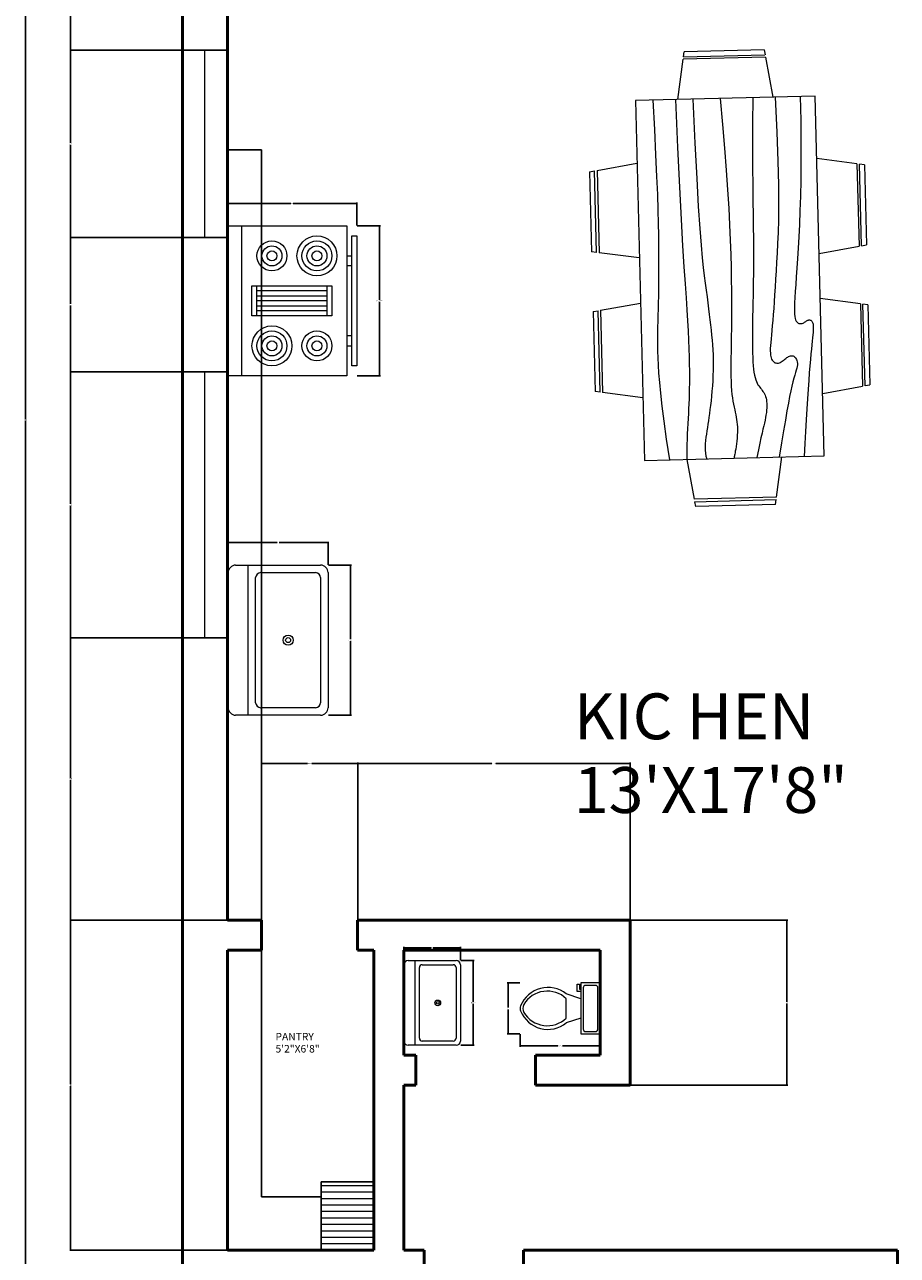
# Model space of a CAD drawing. Units: inches. Extents: x 2208 to 4689, y 1219 to 3512.
# Tile 2 of 5: x 2208 to 2382, y 1383 to 1629. Entities that reach past the tile are written whole.
import ezdxf

# ---------------------------------------------------------------- set-up
doc = ezdxf.new("R2010")
doc.units = ezdxf.units.IN
for name, color, linetype, lineweight in [('A-ANNO-DIMS', 2, 'Continuous', 18), ('A-AREA-IDEN', 7, 'Continuous', 18), ('A-EQPM', 8, 'Continuous', 20), ('A-FLOR-CASE', 9, 'Continuous', 25), ('A-FLOR-FIXT', 9, 'Continuous', 20), ('A-FLOR-PATT', 8, 'Continuous', 13), ('A-FURN', 8, 'Continuous', 18), ('A-GLAZ', 4, 'Continuous', 18), ('A-WALL', 7, 'Continuous', 50)]:
    doc.layers.add(name, color=color, linetype=linetype, lineweight=lineweight)
doc.styles.get("Standard").update_dxf_attribs({"font": 'arial.ttf'})
doc.dimstyles.get("Standard").update_dxf_attribs({"dimtxt": 0.18, "dimasz": 0.18, "dimexe": 0.18, "dimexo": 0.0625, "dimgap": 0.09, "dimtad": 0, "dimtih": 1, "dimtoh": 1, "dimdec": 4, "dimzin": 0, "dimdsep": 46, "dimtxsty": 'Standard', "dimcen": 0.09, "dimadec": 0, "dimazin": 0, "dimtfac": 1, "dimtdec": 4, "dimtofl": 0, "dimtmove": 0, "dimatfit": 3, "dimfxl": 1, "dimtolj": 1, "dimtzin": 0, "dimarcsym": 0})

# ---------------------------------------------------------------- blocks, each defined once
blk = doc.blocks.new('Sink-single - 30 in top')
blk.add_line((-15, -3.999996), (15, -3.999996))
for points in [[(-13.5, 0), (13.5, 0)], [(-15, -18.499996), (-15, -1.5)], [(15, -1.5), (15, -18.499996)], [(-13.5, -17.499996), (-13.5, -6.499996)], [(-12.5, -5.499996), (12.5, -5.499996)], [(13.5, -6.499996), (13.5, -17.499996)], [(12.5, -18.499996), (-12.5, -18.499996)], [(13.5, -19.999996), (-13.5, -19.999996)]]:
    blk.add_lwpolyline(points)
for radius in [1, 0.5]:
    blk.add_circle((0, -11.999996), radius)
for centre, radius, start, end in [((-13.5, -1.5), 1.5, 90, 180), ((13.5, -1.5), 1.5, 0, 90), ((-12.5, -6.499996), 1, 90, 180), ((12.5, -6.499996), 1, 0, 90), ((-13.5, -18.499996), 1.5, 180, 270), ((-12.5, -17.499996), 1, 180, 270), ((12.5, -17.499996), 1, 270, 0), ((13.5, -18.499996), 1.5, 270, 0)]:
    blk.add_arc(centre, radius, start, end)
blk = doc.blocks.new('Range-Oven - 30 in top')
for p, q in [((0, -3), (30, -3)), ((12, -6), (18, -6)), ((13, -20), (13, -6)), ((14, -6), (14, -20)), ((15, -20), (15, -6)), ((16, -6), (16, -20)), ((17, -20), (17, -6)), ((18, -20), (12, -20)), ((6, -24), (6, -25)), ((8, -25), (8, -24)), ((22, -25), (22, -24)), ((24, -24), (24, -25))]:
    blk.add_line(p, q)
for points in [[(0, -24), (0, 0), (30, 0), (30, -24)], [(12, -21), (12, -5), (18, -5), (18, -21)], [(2, -26), (2, -25), (28, -25), (28, -26)]]:
    blk.add_lwpolyline(points, close=True)
for centre, radius in [((6, -9), 4), ((6, -9), 3), ((6, -9), 2), ((24, -9), 3), ((24, -9), 2), ((6, -9), 1), ((24, -9), 1), ((24, -18), 4), ((6, -18), 3), ((6, -18), 2), ((6, -18), 1), ((24, -18), 3), ((24, -18), 2), ((24, -18), 1)]:
    blk.add_circle(centre, radius)
blk = doc.blocks.new('Toilet - top')
for p, q in [((9.5, -6), (9.5, -2)), ((-10, -8.5), (-8, -8.5)), ((-10, -9.5), (-10, -8.5)), ((-7, -9.5), (-10, -9.5)), ((-8, -8.5), (-8, -8)), ((-7, -8), (-7, -9.5)), ((-4, -8), (-6, -14)), ((4, -8), (6, -14)), ((4, -14), (-4, -14))]:
    blk.add_line(p, q)
blk.add_lwpolyline([(10.5, -8), (10.5, 0), (-10.5, 0), (-10.5, -8)], close=True)
for points in [[(-9.5, -2), (-9.5, -6)], [(8.5, -1), (-8.5, -1)], [(-8.5, -7), (8.5, -7)]]:
    blk.add_lwpolyline(points)
for centre, radius, start, end in [((-8.62, -1.88), 0.884, 81.8699, 188.1301), ((8.62, -1.88), 0.884, 351.8699, 98.1301), ((-8.62, -6.12), 0.884, 171.8699, 278.1301), ((8.62, -6.12), 0.884, 261.8699, 8.1301), ((3.52, -21.58), 12.17, 141.4691, 247.9714), ((4.2, -21.82), 11.33, 136.3677, 238.9468), ((-3.52, -21.58), 12.17, 292.0284, 38.5307), ((-4.2, -21.82), 11.33, 301.053, 43.6321), ((0, -27.88), 4, 245.7318, 294.2682), ((0, -29), 4, 254.8605, 285.1395)]:
    blk.add_arc(centre, radius, start, end)
blk = doc.blocks.new('Dining Set - 36 x 72 in.')
for p, q in [((-22, 27.5), (-22.1562, 26.50042)), ((-22, 27.5), (-6, 27.5)), ((-5.8437, 26.49966), (-6, 27.5)), ((6, 27.5), (5.8438, 26.50042)), ((6, 27.5), (22, 27.5)), ((22.1563, 26.49966), (22, 27.5)), ((-22.2343, 26.00059), (-23.4847, 17.99762)), ((-22.2304, 26), (-5.7608, 26)), ((-5.8416, 26.5), (-22.1534, 26.5)), ((-4.5152, 17.99762), (-5.7655, 25.99926)), ((5.7657, 26.00059), (4.5153, 17.99762)), ((5.7696, 26), (22.2392, 26)), ((22.1584, 26.5), (5.8466, 26.5)), ((23.4848, 17.99762), (22.2345, 25.99926)), ((36, 18), (-36, 18)), ((-36, 18), (-36, -18)), ((36, -18), (36, 18)), ((-45.5, 8), (-44.5004, 8.15617)), ((-45.5, 8), (-45.5, -8)), ((-44.5, -8.15843), (-44.5, 8.15338)), ((-44.0006, 8.23428), (-35.9976, 9.48474)), ((-44, 8.23041), (-44, -8.23915)), ((44.0006, 8.23428), (35.9976, 9.48474)), ((44, 8.23041), (44, -8.23915)), ((44.5, -8.15843), (44.5, 8.15338)), ((45.5, 8), (44.5005, 8.15617)), ((45.5, 8), (45.5, -8)), ((-44.4997, -8.15631), (-45.5, -8)), ((-35.9976, -9.48476), (-43.9993, -8.2345)), ((35.9976, -9.48476), (43.9993, -8.2345)), ((44.4997, -8.15631), (45.5, -8)), ((-36, -18), (36, -18)), ((-22.2343, -26.0006), (-23.4847, -17.99762)), ((-4.5152, -17.99762), (-5.7655, -25.99928)), ((5.7657, -26.0006), (4.5153, -17.99762)), ((23.4848, -17.99762), (22.2345, -25.99928)), ((-22.2304, -26), (-5.7608, -26)), ((-22, -27.5), (-22.1562, -26.50044)), ((-5.8416, -26.5), (-22.1534, -26.5)), ((-5.8437, -26.49967), (-6, -27.5)), ((5.7696, -26), (22.2392, -26)), ((6, -27.5), (5.8438, -26.50044)), ((22.1584, -26.5), (5.8466, -26.5)), ((22.1563, -26.49967), (22, -27.5)), ((-22, -27.5), (-6, -27.5)), ((6, -27.5), (22, -27.5))]:
    blk.add_line(p, q)
for points in [[(-36, 15), (-31.1772, 14.97754), (-26.8079, 14.91406), (-22.8538, 14.81543), (-19.276, 14.6875), (-16.0362, 14.53613), (-13.0957, 14.36718), (-10.4159, 14.18652), (-7.9583, 14), (-5.6904, 13.81315), (-3.6035, 13.63021), (-1.6954, 13.45508), (0.0365, 13.29166), (1.5945, 13.14388), (2.9811, 13.01562), (4.1988, 12.9108), (5.25, 12.83333), (6.1393, 12.78613), (6.8802, 12.76823), (7.4883, 12.77767), (7.9792, 12.8125), (8.3685, 12.87077), (8.6719, 12.95052), (8.9049, 13.0498), (9.0833, 13.16666), (9.2205, 13.29899), (9.3216, 13.44401), (9.3895, 13.59879), (9.4271, 13.76041), (9.4373, 13.92594), (9.4232, 14.09245), (9.3875, 14.257), (9.3333, 14.41666), (9.2638, 14.56917), (9.1836, 14.71484), (9.0975, 14.85465), (9.0104, 14.98958), (8.9272, 15.1206), (8.8529, 15.2487), (8.7922, 15.37483), (8.75, 15.5), (8.7305, 15.62467), (8.7344, 15.74739), (8.7617, 15.86621), (8.8125, 15.97916), (8.8867, 16.08431), (8.9844, 16.17968), (9.1055, 16.26334), (9.25, 16.33333), (9.4189, 16.38802), (9.6172, 16.42708), (9.8506, 16.45052), (10.125, 16.45833), (10.4463, 16.45052), (10.8203, 16.42708), (11.2529, 16.38802), (11.75, 16.33333), (12.3184, 16.26318), (12.9694, 16.17838), (13.7151, 16.07991), (14.5677, 15.96875), (15.5395, 15.84586), (16.6426, 15.71224), (17.8893, 15.56884), (19.2917, 15.41666), (20.859, 15.25667), (22.5879, 15.08984), (24.4721, 14.91715), (26.5052, 14.73958), (28.6809, 14.5581), (30.9929, 14.3737), (33.4347, 14.18733), (36, 14)], [(-36, 10), (-28.9766, 10.14274), (-23.1725, 10.20442), (-18.4241, 10.19775), (-14.5677, 10.13541), (-11.4399, 10.03011), (-8.877, 9.89453), (-6.7154, 9.74137), (-4.7917, 9.58333), (-2.9698, 9.43082), (-1.2246, 9.28515), (0.4415, 9.14534), (2.026, 9.01041), (3.5266, 8.87939), (4.9408, 8.7513), (6.266, 8.62516), (7.5, 8.5), (8.6411, 8.37549), (9.6914, 8.2539), (10.6538, 8.13818), (11.5312, 8.03125), (12.3267, 7.93603), (13.043, 7.85547), (13.6831, 7.79248), (14.25, 7.75), (14.7471, 7.7303), (15.1797, 7.73307), (15.5537, 7.75732), (15.875, 7.80208), (16.1494, 7.86637), (16.3828, 7.94922), (16.5811, 8.04964), (16.75, 8.16666), (16.8944, 8.29915), (17.0143, 8.44531), (17.1089, 8.60319), (17.1771, 8.77083), (17.218, 8.94629), (17.2305, 9.1276), (17.2137, 9.31282), (17.1667, 9.5), (17.0895, 9.6875), (16.987, 9.875), (16.8649, 10.0625), (16.7292, 10.25), (16.5856, 10.4375), (16.4401, 10.625), (16.2985, 10.8125), (16.1667, 11), (16.05, 11.18733), (15.9518, 11.3737), (15.8752, 11.5581), (15.8229, 11.73958), (15.798, 11.91715), (15.8034, 12.08984), (15.842, 12.25667), (15.9167, 12.41666), (16.0295, 12.56836), (16.1784, 12.70833), (16.3605, 12.83268), (16.5729, 12.9375), (16.8127, 13.01888), (17.0768, 13.07291), (17.3625, 13.0957), (17.6667, 13.08333), (17.9894, 13.03312), (18.3418, 12.94726), (18.7382, 12.82918), (19.1927, 12.68229), (19.7195, 12.51001), (20.3327, 12.31575), (21.0465, 12.10294), (21.875, 11.875), (22.8357, 11.63354), (23.959, 11.37304), (25.2786, 11.08618), (26.8282, 10.76562), (28.6414, 10.40405), (30.752, 9.99414), (33.1936, 9.52856), (36, 9)], [(-36, 5.5), (-30.7157, 5.3348), (-26.069, 5.20963), (-21.9946, 5.11767), (-18.4271, 5.05208), (-15.3009, 5.00602), (-12.5508, 4.97265), (-10.1112, 4.94515), (-7.9167, 4.91666), (-5.909, 4.88167), (-4.0586, 4.83984), (-2.3429, 4.79215), (-0.7396, 4.73958), (0.7739, 4.6831), (2.22, 4.6237), (3.6213, 4.56233), (5, 4.5), (6.373, 4.43782), (7.7344, 4.3776), (9.0723, 4.32129), (10.375, 4.27083), (11.6309, 4.22819), (12.8281, 4.19531), (13.9551, 4.17415), (15, 4.16666), (15.954, 4.17448), (16.819, 4.19791), (17.6001, 4.23698), (18.3021, 4.29166), (18.9299, 4.36198), (19.4883, 4.44791), (19.9823, 4.54948), (20.4167, 4.66666), (20.7969, 4.79899), (21.1302, 4.94401), (21.4245, 5.09879), (21.6875, 5.26041), (21.9271, 5.42594), (22.1511, 5.59245), (22.3672, 5.757), (22.5834, 5.91666), (22.8065, 6.06868), (23.0404, 6.21093), (23.2879, 6.34147), (23.5521, 6.45833), (23.8358, 6.55957), (24.142, 6.64323), (24.4735, 6.70735), (24.8334, 6.75), (25.2235, 6.76969), (25.642, 6.76692), (26.0858, 6.74267), (26.5521, 6.69791), (27.0379, 6.63362), (27.5404, 6.55078), (28.0565, 6.45036), (28.5834, 6.33333), (29.1242, 6.19987), (29.7071, 6.04687), (30.3661, 5.87044), (31.1354, 5.66666), (32.0493, 5.43164), (33.142, 5.16146), (34.4475, 4.85221), (36, 4.5)], [(-36, -1), (-30.7915, -0.6591), (-26.0195, -0.38216), (-21.6519, -0.16284), (-17.6563, 0.00521), (-14.0005, 0.12833), (-10.6523, 0.21289), (-7.5796, 0.26522), (-4.75, 0.29166), (-2.134, 0.29793), (0.2878, 0.28711), (2.5317, 0.26163), (4.6146, 0.22396), (6.5529, 0.17651), (8.3633, 0.12174), (10.0623, 0.06209), (11.6667, 0), (13.1899, -0.06201), (14.6341, -0.1211), (15.9982, -0.17432), (17.2813, -0.21875), (18.4823, -0.25147), (19.6003, -0.26953), (20.6343, -0.27002), (21.5834, -0.25), (22.4481, -0.20768), (23.2357, -0.14584), (23.9549, -0.06836), (24.6146, 0.02083), (25.2235, 0.11784), (25.7904, 0.21875), (26.3241, 0.31966), (26.8334, 0.41666), (27.3265, 0.50618), (27.8099, 0.58593), (28.2894, 0.65397), (28.7709, 0.70833), (29.2601, 0.74707), (29.763, 0.76823), (30.2855, 0.76985), (30.8334, 0.75), (31.4088, 0.70784), (31.9994, 0.64713), (32.589, 0.57275), (33.1615, 0.48958), (33.7008, 0.4025), (34.1908, 0.3164), (34.6153, 0.23616), (34.9584, 0.16666), (35.2099, 0.11165), (35.3848, 0.07031), (35.504, 0.04069), (35.5886, 0.02083), (35.6594, 0.00879), (35.7377, 0.0026), (35.8442, 0.00032), (36, 0)], [(-36, -6.5), (-27.1843, -6.31267), (-20.084, -6.1263), (-14.469, -5.9419), (-10.1094, -5.76042), (-6.7752, -5.58285), (-4.2363, -5.41016), (-2.2629, -5.24333), (-0.625, -5.08334), (0.8708, -4.93099), (2.2715, -4.78646), (3.5872, -4.64974), (4.8281, -4.52084), (6.0046, -4.39974), (7.127, -4.28646), (8.2053, -4.18099), (9.25, -4.08334), (10.2705, -3.99382), (11.2734, -3.91407), (12.2647, -3.84603), (13.25, -3.79167), (14.2354, -3.75293), (15.2266, -3.73177), (16.2295, -3.73015), (17.25, -3.75), (18.2912, -3.79248), (19.3451, -3.85547), (20.4009, -3.93604), (21.4479, -4.03125), (22.4754, -4.13819), (23.4727, -4.25391), (24.4289, -4.37549), (25.3334, -4.5), (26.1785, -4.62492), (26.9694, -4.74935), (27.7145, -4.87281), (28.4219, -4.99479), (29.1, -5.11483), (29.7572, -5.23242), (30.4016, -5.34709), (31.0417, -5.45834), (31.6837, -5.56437), (32.3262, -5.65821), (32.9658, -5.73153), (33.599, -5.77604), (34.2224, -5.78345), (34.8327, -5.74545), (35.4264, -5.65373), (36, -5.5)], [(-36, -10), (-26.4022, -9.81299), (-18.4675, -9.62891), (-11.9839, -9.45069), (-6.7396, -9.28125), (-2.5226, -9.12354), (0.8789, -8.98047), (3.6769, -8.85498), (6.0833, -8.75), (8.2767, -8.66765), (10.3021, -8.60677), (12.1712, -8.56543), (13.8958, -8.54167), (15.4876, -8.53353), (16.9583, -8.53907), (18.3197, -8.55632), (19.5834, -8.58334), (20.7616, -8.61841), (21.8685, -8.66081), (22.9188, -8.71004), (23.9271, -8.76563), (24.9081, -8.82707), (25.8763, -8.89388), (26.8465, -8.96558), (27.8334, -9.04167), (28.8474, -9.12118), (29.8828, -9.20117), (30.93, -9.27824), (31.9792, -9.34896), (33.0205, -9.40991), (34.0443, -9.45768), (35.0407, -9.48885), (36, -9.5)], [(-36, -14.5), (-30.0881, -14.33513), (-25.0332, -14.21224), (-20.7312, -14.12647), (-17.0781, -14.07292), (-13.97, -14.04671), (-11.3027, -14.04297), (-8.9724, -14.05681), (-6.875, -14.08334), (-4.9224, -14.11833), (-3.0905, -14.16016), (-1.3709, -14.20785), (0.2448, -14.26042), (1.7647, -14.3169), (3.1973, -14.3763), (4.5507, -14.43767), (5.8333, -14.5), (7.0554, -14.5621), (8.235, -14.62175), (9.3922, -14.67652), (10.5469, -14.72396), (11.7192, -14.76164), (12.929, -14.78711), (14.1965, -14.79794), (15.5417, -14.79167), (16.9933, -14.76424), (18.6152, -14.70508), (20.4804, -14.60197), (22.6615, -14.44271), (25.2312, -14.21509), (28.2624, -13.9069), (31.8277, -13.50594), (36, -13)]]:
    blk.add_lwpolyline(points)
blk = doc.blocks.new('*D22')
at = {"layer": 'A-ANNO-DIMS', "color": 0, "lineweight": -2, "transparency": 16777216}
for p, q in [((2268.33, 1521.37), (2272.94, 1521.37)), ((2272.76, 1521.19), (2272.76, 1506.55)), ((2272.76, 1491.55), (2272.76, 1506.18)), ((2268.33, 1491.37), (2272.94, 1491.37))]:
    blk.add_line(p, q, dxfattribs=at)
at = {"layer": 'A-ANNO-DIMS', "color": 0, "transparency": 16777216}
for points in [[(2272.73, 1521.19), (2272.79, 1521.19), (2272.76, 1521.37)], [(2272.73, 1491.55), (2272.79, 1491.55), (2272.76, 1491.37)]]:
    blk.add_solid(points, dxfattribs=at)
at = {"layer": 'Defpoints', "color": 0, "transparency": 16777216}
for p in [(2268.26, 1521.37), (2272.76, 1521.37), (2268.26, 1491.37)]:
    blk.add_point(p, dxfattribs=at)
at = {"layer": 'A-ANNO-DIMS', "color": 0, "transparency": 16777216, "insert": (2272.76, 1506.37), "char_height": 0.18, "attachment_point": 5}
blk.add_mtext('\\A1;SINK 30', dxfattribs=at)
blk = doc.blocks.new('*D23')
at = {"layer": 'A-ANNO-DIMS', "color": 0, "lineweight": -2, "transparency": 16777216}
for p, q in [((2248.26, 1521.43), (2248.26, 1526.05)), ((2248.44, 1525.87), (2258.04, 1525.87)), ((2268.08, 1525.87), (2258.48, 1525.87)), ((2268.26, 1521.43), (2268.26, 1526.05))]:
    blk.add_line(p, q, dxfattribs=at)
at = {"layer": 'A-ANNO-DIMS', "color": 0, "transparency": 16777216}
for points in [[(2248.44, 1525.9), (2248.44, 1525.84), (2248.26, 1525.87)], [(2268.08, 1525.9), (2268.08, 1525.84), (2268.26, 1525.87)]]:
    blk.add_solid(points, dxfattribs=at)
at = {"layer": 'Defpoints', "color": 0, "transparency": 16777216}
for p in [(2248.26, 1525.87), (2248.26, 1521.37), (2268.26, 1521.37)]:
    blk.add_point(p, dxfattribs=at)
at = {"layer": 'A-ANNO-DIMS', "color": 0, "transparency": 16777216, "insert": (2258.26, 1525.87), "char_height": 0.18, "attachment_point": 5}
blk.add_mtext('\\A1;20', dxfattribs=at)
blk = doc.blocks.new('*D24')
at = {"layer": 'A-ANNO-DIMS', "color": 0, "lineweight": -2, "transparency": 16777216}
for p, q in [((2294.78, 1442.31), (2297.44, 1442.31)), ((2297.26, 1442.13), (2297.26, 1434.01)), ((2297.26, 1425.53), (2297.26, 1433.65)), ((2294.78, 1425.35), (2297.44, 1425.35))]:
    blk.add_line(p, q, dxfattribs=at)
at = {"layer": 'A-ANNO-DIMS', "color": 0, "transparency": 16777216}
for points in [[(2297.23, 1442.13), (2297.29, 1442.13), (2297.26, 1442.31)], [(2297.23, 1425.53), (2297.29, 1425.53), (2297.26, 1425.35)]]:
    blk.add_solid(points, dxfattribs=at)
at = {"layer": 'Defpoints', "color": 0, "transparency": 16777216}
for p in [(2294.71, 1442.31), (2297.26, 1442.31), (2294.71, 1425.35)]:
    blk.add_point(p, dxfattribs=at)
at = {"layer": 'A-ANNO-DIMS', "color": 0, "transparency": 16777216, "insert": (2297.26, 1433.83), "char_height": 0.18, "attachment_point": 5}
blk.add_mtext('\\A1;SINK 17', dxfattribs=at)
blk = doc.blocks.new('*D25')
at = {"layer": 'A-ANNO-DIMS', "color": 0, "lineweight": -2, "transparency": 16777216}
for p, q in [((2283.4, 1442.38), (2283.4, 1445.04)), ((2294.71, 1442.38), (2294.71, 1445.04)), ((2283.58, 1444.86), (2288.87, 1444.86)), ((2294.53, 1444.86), (2289.25, 1444.86))]:
    blk.add_line(p, q, dxfattribs=at)
at = {"layer": 'A-ANNO-DIMS', "color": 0, "transparency": 16777216}
for points in [[(2283.58, 1444.89), (2283.58, 1444.83), (2283.4, 1444.86)], [(2294.53, 1444.89), (2294.53, 1444.83), (2294.71, 1444.86)]]:
    blk.add_solid(points, dxfattribs=at)
at = {"layer": 'Defpoints', "color": 0, "transparency": 16777216}
for p in [(2283.4, 1444.86), (2283.4, 1442.31), (2294.71, 1442.31)]:
    blk.add_point(p, dxfattribs=at)
at = {"layer": 'A-ANNO-DIMS', "color": 0, "transparency": 16777216, "insert": (2289.06, 1444.86), "char_height": 0.18, "attachment_point": 5}
blk.add_mtext('\\A1;11', dxfattribs=at)
blk = doc.blocks.new('*D28')
at = {"layer": 'A-ANNO-DIMS', "color": 0, "lineweight": -2, "transparency": 16777216}
for p, q in [((2274.09, 1589.22), (2278.71, 1589.22)), ((2278.53, 1589.04), (2278.53, 1574.41)), ((2278.53, 1559.4), (2278.53, 1574.04)), ((2274.09, 1559.22), (2278.71, 1559.22))]:
    blk.add_line(p, q, dxfattribs=at)
at = {"layer": 'A-ANNO-DIMS', "color": 0, "transparency": 16777216}
for points in [[(2278.5, 1589.04), (2278.56, 1589.04), (2278.53, 1589.22)], [(2278.5, 1559.4), (2278.56, 1559.4), (2278.53, 1559.22)]]:
    blk.add_solid(points, dxfattribs=at)
at = {"layer": 'Defpoints', "color": 0, "transparency": 16777216}
for p in [(2274.03, 1589.22), (2278.53, 1589.22), (2274.03, 1559.22)]:
    blk.add_point(p, dxfattribs=at)
at = {"layer": 'A-ANNO-DIMS', "color": 0, "transparency": 16777216, "insert": (2278.53, 1574.22), "char_height": 0.18, "attachment_point": 5}
blk.add_mtext('\\A1;RANGE 30', dxfattribs=at)
blk = doc.blocks.new('*D29')
at = {"layer": 'A-ANNO-DIMS', "color": 0, "lineweight": -2, "transparency": 16777216}
for p, q in [((2248.03, 1589.29), (2248.03, 1593.9)), ((2248.21, 1593.72), (2260.81, 1593.72)), ((2273.85, 1593.72), (2261.25, 1593.72)), ((2274.03, 1589.29), (2274.03, 1593.9))]:
    blk.add_line(p, q, dxfattribs=at)
at = {"layer": 'A-ANNO-DIMS', "color": 0, "transparency": 16777216}
for points in [[(2248.21, 1593.75), (2248.21, 1593.69), (2248.03, 1593.72)], [(2273.85, 1593.75), (2273.85, 1593.69), (2274.03, 1593.72)]]:
    blk.add_solid(points, dxfattribs=at)
at = {"layer": 'Defpoints', "color": 0, "transparency": 16777216}
for p in [(2248.03, 1593.72), (2248.03, 1589.22), (2274.03, 1589.22)]:
    blk.add_point(p, dxfattribs=at)
at = {"layer": 'A-ANNO-DIMS', "color": 0, "transparency": 16777216, "insert": (2261.03, 1593.72), "char_height": 0.18, "attachment_point": 5}
blk.add_mtext('\\A1;26', dxfattribs=at)
blk = doc.blocks.new('*D30')
at = {"layer": 'A-ANNO-DIMS', "color": 0, "lineweight": -2, "transparency": 16777216}
for p, q in [((2306.67, 1427.56), (2306.67, 1425.04)), ((2306.85, 1425.22), (2314.21, 1425.22)), ((2322.51, 1425.22), (2315.15, 1425.22)), ((2322.69, 1427.56), (2322.69, 1425.04))]:
    blk.add_line(p, q, dxfattribs=at)
at = {"layer": 'A-ANNO-DIMS', "color": 0, "transparency": 16777216}
for points in [[(2306.85, 1425.25), (2306.85, 1425.19), (2306.67, 1425.22)], [(2322.51, 1425.25), (2322.51, 1425.19), (2322.69, 1425.22)]]:
    blk.add_solid(points, dxfattribs=at)
at = {"layer": 'Defpoints', "color": 0, "transparency": 16777216}
for p in [(2306.67, 1427.62), (2322.69, 1427.62), (2322.69, 1425.22)]:
    blk.add_point(p, dxfattribs=at)
at = {"layer": 'A-ANNO-DIMS', "color": 0, "transparency": 16777216, "insert": (2314.68, 1425.22), "char_height": 0.18, "attachment_point": 5}
blk.add_mtext('\\A1;WC 16', dxfattribs=at)
blk = doc.blocks.new('*D31')
at = {"layer": 'A-ANNO-DIMS', "color": 0, "lineweight": -2, "transparency": 16777216}
for p, q in [((2306.61, 1437.81), (2304.08, 1437.81)), ((2304.26, 1437.63), (2304.26, 1432.9)), ((2304.26, 1427.8), (2304.26, 1432.53)), ((2306.61, 1427.62), (2304.08, 1427.62))]:
    blk.add_line(p, q, dxfattribs=at)
at = {"layer": 'A-ANNO-DIMS', "color": 0, "transparency": 16777216}
for points in [[(2304.23, 1437.63), (2304.29, 1437.63), (2304.26, 1437.81)], [(2304.23, 1427.8), (2304.29, 1427.8), (2304.26, 1427.62)]]:
    blk.add_solid(points, dxfattribs=at)
at = {"layer": 'Defpoints', "color": 0, "transparency": 16777216}
for p in [(2306.67, 1437.81), (2304.26, 1427.62), (2306.67, 1427.62)]:
    blk.add_point(p, dxfattribs=at)
at = {"layer": 'A-ANNO-DIMS', "color": 0, "transparency": 16777216, "insert": (2304.26, 1432.72), "char_height": 0.18, "attachment_point": 5}
blk.add_mtext('\\A1;10', dxfattribs=at)
blk = doc.blocks.new('*D35')
at = {"layer": 'A-ANNO-DIMS', "color": 0, "lineweight": -2, "transparency": 16777216}
for p, q in [((2239.04, 1850.36), (2207.57, 1850.36)), ((2207.75, 1850.18), (2207.75, 1550.54)), ((2207.75, 1250.54), (2207.75, 1550.17)), ((2239.04, 1250.36), (2207.57, 1250.36))]:
    blk.add_line(p, q, dxfattribs=at)
at = {"layer": 'A-ANNO-DIMS', "color": 0, "transparency": 16777216}
for points in [[(2207.72, 1850.18), (2207.78, 1850.18), (2207.75, 1850.36)], [(2207.72, 1250.54), (2207.78, 1250.54), (2207.75, 1250.36)]]:
    blk.add_solid(points, dxfattribs=at)
at = {"layer": 'Defpoints', "color": 0, "transparency": 16777216}
for p in [(2207.75, 1850.36), (2239.1, 1850.36), (2239.1, 1250.36)]:
    blk.add_point(p, dxfattribs=at)
at = {"layer": 'A-ANNO-DIMS', "color": 0, "transparency": 16777216, "insert": (2207.75, 1550.36), "char_height": 0.18, "attachment_point": 5}
blk.add_mtext('\\A1;600', dxfattribs=at)
blk = doc.blocks.new('*D41')
at = {"layer": 'A-ANNO-DIMS', "color": 0, "lineweight": -2, "transparency": 16777216}
for p, q in [((2248.04, 1450.36), (2216.57, 1450.36)), ((2216.75, 1450.18), (2216.75, 1417.54)), ((2216.75, 1384.54), (2216.75, 1417.17)), ((2248.04, 1384.36), (2216.57, 1384.36))]:
    blk.add_line(p, q, dxfattribs=at)
at = {"layer": 'A-ANNO-DIMS', "color": 0, "transparency": 16777216}
for points in [[(2216.72, 1450.18), (2216.78, 1450.18), (2216.75, 1450.36)], [(2216.72, 1384.54), (2216.78, 1384.54), (2216.75, 1384.36)]]:
    blk.add_solid(points, dxfattribs=at)
at = {"layer": 'Defpoints', "color": 0, "transparency": 16777216}
for p in [(2216.75, 1450.36), (2248.1, 1450.36), (2248.1, 1384.36)]:
    blk.add_point(p, dxfattribs=at)
at = {"layer": 'A-ANNO-DIMS', "color": 0, "transparency": 16777216, "insert": (2216.75, 1417.36), "char_height": 0.18, "attachment_point": 5}
blk.add_mtext('\\A1;66', dxfattribs=at)
blk = doc.blocks.new('*D42')
at = {"layer": 'A-ANNO-DIMS', "color": 0, "lineweight": -2, "transparency": 16777216}
for p, q in [((2248.04, 1506.86), (2216.57, 1506.86)), ((2216.75, 1506.68), (2216.75, 1478.79)), ((2216.75, 1450.54), (2216.75, 1478.43)), ((2248.04, 1450.36), (2216.57, 1450.36))]:
    blk.add_line(p, q, dxfattribs=at)
at = {"layer": 'A-ANNO-DIMS', "color": 0, "transparency": 16777216}
for points in [[(2216.72, 1506.68), (2216.78, 1506.68), (2216.75, 1506.86)], [(2216.72, 1450.54), (2216.78, 1450.54), (2216.75, 1450.36)]]:
    blk.add_solid(points, dxfattribs=at)
at = {"layer": 'Defpoints', "color": 0, "transparency": 16777216}
for p in [(2216.75, 1506.86), (2248.1, 1506.86), (2248.1, 1450.36)]:
    blk.add_point(p, dxfattribs=at)
at = {"layer": 'A-ANNO-DIMS', "color": 0, "transparency": 16777216, "insert": (2216.75, 1478.61), "char_height": 0.18, "attachment_point": 5}
blk.add_mtext('\\A1;56.51', dxfattribs=at)
blk = doc.blocks.new('*D43')
at = {"layer": 'A-ANNO-DIMS', "color": 0, "lineweight": -2, "transparency": 16777216}
for p, q in [((2248.04, 1560.01), (2216.57, 1560.01)), ((2216.75, 1559.83), (2216.75, 1533.62)), ((2216.75, 1507.04), (2216.75, 1533.26)), ((2248.04, 1506.86), (2216.57, 1506.86))]:
    blk.add_line(p, q, dxfattribs=at)
at = {"layer": 'A-ANNO-DIMS', "color": 0, "transparency": 16777216}
for points in [[(2216.72, 1559.83), (2216.78, 1559.83), (2216.75, 1560.01)], [(2216.72, 1507.04), (2216.78, 1507.04), (2216.75, 1506.86)]]:
    blk.add_solid(points, dxfattribs=at)
at = {"layer": 'Defpoints', "color": 0, "transparency": 16777216}
for p in [(2216.75, 1560.01), (2248.1, 1560.01), (2248.1, 1506.86)]:
    blk.add_point(p, dxfattribs=at)
at = {"layer": 'A-ANNO-DIMS', "color": 0, "transparency": 16777216, "insert": (2216.75, 1533.44), "char_height": 0.18, "attachment_point": 5}
blk.add_mtext('\\A1;53.15', dxfattribs=at)
blk = doc.blocks.new('*D44')
at = {"layer": 'A-ANNO-DIMS', "color": 0, "lineweight": -2, "transparency": 16777216}
for p, q in [((2248.04, 1586.91), (2216.57, 1586.91)), ((2216.75, 1586.73), (2216.75, 1573.64)), ((2216.75, 1560.19), (2216.75, 1573.28)), ((2248.04, 1560.01), (2216.57, 1560.01))]:
    blk.add_line(p, q, dxfattribs=at)
at = {"layer": 'A-ANNO-DIMS', "color": 0, "transparency": 16777216}
for points in [[(2216.72, 1586.73), (2216.78, 1586.73), (2216.75, 1586.91)], [(2216.72, 1560.19), (2216.78, 1560.19), (2216.75, 1560.01)]]:
    blk.add_solid(points, dxfattribs=at)
at = {"layer": 'Defpoints', "color": 0, "transparency": 16777216}
for p in [(2216.75, 1586.91), (2248.1, 1586.91), (2248.1, 1560.01)]:
    blk.add_point(p, dxfattribs=at)
at = {"layer": 'A-ANNO-DIMS', "color": 0, "transparency": 16777216, "insert": (2216.75, 1573.46), "char_height": 0.18, "attachment_point": 5}
blk.add_mtext('\\A1;26.9', dxfattribs=at)
blk = doc.blocks.new('*D45')
at = {"layer": 'A-ANNO-DIMS', "color": 0, "lineweight": -2, "transparency": 16777216}
for p, q in [((2248.04, 1624.35), (2216.57, 1624.35)), ((2216.75, 1624.17), (2216.75, 1605.81)), ((2216.75, 1587.09), (2216.75, 1605.45)), ((2248.04, 1586.91), (2216.57, 1586.91))]:
    blk.add_line(p, q, dxfattribs=at)
at = {"layer": 'A-ANNO-DIMS', "color": 0, "transparency": 16777216}
for points in [[(2216.72, 1624.17), (2216.78, 1624.17), (2216.75, 1624.35)], [(2216.72, 1587.09), (2216.78, 1587.09), (2216.75, 1586.91)]]:
    blk.add_solid(points, dxfattribs=at)
at = {"layer": 'Defpoints', "color": 0, "transparency": 16777216}
for p in [(2216.75, 1624.35), (2248.1, 1624.35), (2248.1, 1586.91)]:
    blk.add_point(p, dxfattribs=at)
at = {"layer": 'A-ANNO-DIMS', "color": 0, "transparency": 16777216, "insert": (2216.75, 1605.63), "char_height": 0.18, "attachment_point": 5}
blk.add_mtext('\\A1;37.44', dxfattribs=at)
blk = doc.blocks.new('*D46')
at = {"layer": 'A-ANNO-DIMS', "color": 0, "lineweight": -2, "transparency": 16777216}
for p, q in [((2248.04, 1841.36), (2216.57, 1841.36)), ((2216.75, 1841.18), (2216.75, 1733.03)), ((2216.75, 1624.53), (2216.75, 1732.67)), ((2248.04, 1624.35), (2216.57, 1624.35))]:
    blk.add_line(p, q, dxfattribs=at)
at = {"layer": 'A-ANNO-DIMS', "color": 0, "transparency": 16777216}
for points in [[(2216.72, 1841.18), (2216.78, 1841.18), (2216.75, 1841.36)], [(2216.72, 1624.53), (2216.78, 1624.53), (2216.75, 1624.35)]]:
    blk.add_solid(points, dxfattribs=at)
at = {"layer": 'Defpoints', "color": 0, "transparency": 16777216}
for p in [(2216.75, 1841.36), (2248.1, 1841.36), (2248.1, 1624.35)]:
    blk.add_point(p, dxfattribs=at)
at = {"layer": 'A-ANNO-DIMS', "color": 0, "transparency": 16777216, "insert": (2216.75, 1732.85), "char_height": 0.18, "attachment_point": 5}
blk.add_mtext('\\A1;217', dxfattribs=at)
blk = doc.blocks.new('*D67')
at = {"layer": 'A-ANNO-DIMS', "color": 0, "lineweight": -2, "transparency": 16777216}
for p, q in [((2254.94, 1450.42), (2254.94, 1481.89)), ((2274.17, 1450.42), (2274.17, 1481.89)), ((2255.12, 1481.71), (2264.1, 1481.71)), ((2273.99, 1481.71), (2265.01, 1481.71))]:
    blk.add_line(p, q, dxfattribs=at)
at = {"layer": 'A-ANNO-DIMS', "color": 0, "transparency": 16777216}
for points in [[(2255.12, 1481.74), (2255.12, 1481.68), (2254.94, 1481.71)], [(2273.99, 1481.74), (2273.99, 1481.68), (2274.17, 1481.71)]]:
    blk.add_solid(points, dxfattribs=at)
at = {"layer": 'Defpoints', "color": 0, "transparency": 16777216}
for p in [(2274.17, 1481.71), (2254.94, 1450.36), (2274.17, 1450.36)]:
    blk.add_point(p, dxfattribs=at)
at = {"layer": 'A-ANNO-DIMS', "color": 0, "transparency": 16777216, "insert": (2264.55, 1481.71), "char_height": 0.18, "attachment_point": 5}
blk.add_mtext('\\A1;19.228', dxfattribs=at)
blk = doc.blocks.new('*D68')
at = {"layer": 'A-ANNO-DIMS', "color": 0, "lineweight": -2, "transparency": 16777216}
for p, q in [((2274.17, 1450.42), (2274.17, 1481.89)), ((2328.69, 1450.42), (2328.69, 1481.89)), ((2274.35, 1481.71), (2301.03, 1481.71)), ((2328.51, 1481.71), (2301.82, 1481.71))]:
    blk.add_line(p, q, dxfattribs=at)
at = {"layer": 'A-ANNO-DIMS', "color": 0, "transparency": 16777216}
for points in [[(2274.35, 1481.74), (2274.35, 1481.68), (2274.17, 1481.71)], [(2328.51, 1481.74), (2328.51, 1481.68), (2328.69, 1481.71)]]:
    blk.add_solid(points, dxfattribs=at)
at = {"layer": 'Defpoints', "color": 0, "transparency": 16777216}
for p in [(2328.69, 1481.71), (2274.17, 1450.36), (2328.69, 1450.36)]:
    blk.add_point(p, dxfattribs=at)
at = {"layer": 'A-ANNO-DIMS', "color": 0, "transparency": 16777216, "insert": (2301.43, 1481.71), "char_height": 0.18, "attachment_point": 5}
blk.add_mtext('\\A1;54.53', dxfattribs=at)
blk = doc.blocks.new('*D69')
at = {"layer": 'A-ANNO-DIMS', "color": 0, "lineweight": -2, "transparency": 16777216}
for p, q in [((2328.75, 1450.36), (2360.22, 1450.36)), ((2360.04, 1450.18), (2360.04, 1434.04)), ((2360.04, 1417.54), (2360.04, 1433.67)), ((2328.75, 1417.36), (2360.22, 1417.36))]:
    blk.add_line(p, q, dxfattribs=at)
at = {"layer": 'A-ANNO-DIMS', "color": 0, "transparency": 16777216}
for points in [[(2360.01, 1450.18), (2360.07, 1450.18), (2360.04, 1450.36)], [(2360.01, 1417.54), (2360.07, 1417.54), (2360.04, 1417.36)]]:
    blk.add_solid(points, dxfattribs=at)
at = {"layer": 'Defpoints', "color": 0, "transparency": 16777216}
for p in [(2328.69, 1450.36), (2328.69, 1417.36), (2360.04, 1417.36)]:
    blk.add_point(p, dxfattribs=at)
at = {"layer": 'A-ANNO-DIMS', "color": 0, "transparency": 16777216, "insert": (2360.04, 1433.86), "char_height": 0.18, "attachment_point": 5}
blk.add_mtext('\\A1;33', dxfattribs=at)

msp = doc.modelspace()

# ---------------------------------------------------------------- hatches: boundary and pattern name
at = {"layer": 'A-FLOR-PATT'}
h = msp.add_hatch(dxfattribs=at)
h.set_pattern_fill('ANSI31', color=256, scale=0.407119, angle=-45, style=0)
h.paths.add_polyline_path([(2266.8602, 1384.3551), (2277.3743, 1384.3551), (2277.3743, 1398.0664), (2266.8602, 1398.0664)])

# ---------------------------------------------------------------- linework, layer by layer
at = {"layer": 'A-FLOR-CASE'}
for p, q in [((2254.938, 1604.4172), (2248.0983, 1604.4172)), ((2254.938, 1450.3551), (2254.938, 1604.4172)), ((2254.938, 1444.3551), (2254.938, 1395.0026)), ((2266.8602, 1395.0026), (2266.8602, 1398.0664)), ((2266.8602, 1398.0664), (2277.3743, 1398.0664)), ((2277.3743, 1398.0664), (2277.3743, 1396.5739)), ((2254.938, 1395.0026), (2266.8602, 1395.0026)), ((2266.8602, 1395.0026), (2266.8602, 1384.3551)), ((2277.3743, 1393.9112), (2277.3743, 1392.264)), ((2266.8602, 1392.264), (2266.8602, 1389.6788)), ((2266.8602, 1388.4271), (2266.8602, 1390.9714)), ((2277.3743, 1390.9714), (2277.3743, 1393.0876)), ((2277.3743, 1389.6788), (2277.3743, 1387.1753)), ((2277.3743, 1385.5575), (2277.3743, 1388.4271)), ((2266.8602, 1387.1753), (2266.8602, 1385.5575))]:
    msp.add_line(p, q, dxfattribs=at)
at = {"layer": 'A-GLAZ'}
for p, q in [((2248.0983, 1624.3486), (2239.0983, 1624.3486)), ((2243.5983, 1586.9092), (2243.5983, 1624.3486)), ((2243.5983, 1624.3486), (2248.0983, 1624.3486)), ((2248.0983, 1586.9092), (2239.0983, 1586.9092)), ((2248.0983, 1560.0107), (2239.0983, 1560.0107)), ((2243.5983, 1506.8648), (2243.5983, 1560.0107)), ((2243.5983, 1560.0107), (2248.0983, 1560.0107)), ((2248.0983, 1506.8648), (2239.0983, 1506.8648))]:
    msp.add_line(p, q, dxfattribs=at)
at = {"layer": 'A-WALL'}
for p, q in [((2239.0983, 1850.3551), (2239.0983, 1250.3551)), ((2248.0983, 1841.3551), (2248.0983, 1450.3551)), ((2254.938, 1450.3551), (2248.0983, 1450.3551)), ((2254.938, 1450.3551), (2254.938, 1444.3551)), ((2283.3743, 1450.3551), (2274.1656, 1450.3551)), ((2274.1656, 1444.3551), (2274.1656, 1450.3551)), ((2328.6911, 1450.3551), (2283.3743, 1450.3551)), ((2328.6911, 1417.3551), (2328.6911, 1450.3551)), ((2248.0983, 1444.3551), (2248.0983, 1384.3551)), ((2254.938, 1444.3551), (2248.0983, 1444.3551)), ((2277.3743, 1444.3551), (2274.1656, 1444.3551)), ((2277.3743, 1384.3551), (2277.3743, 1444.3551)), ((2322.6911, 1444.3551), (2283.3743, 1444.3551)), ((2283.3743, 1423.3551), (2283.3743, 1444.3551)), ((2322.6911, 1423.3551), (2322.6911, 1444.3551)), ((2283.3743, 1423.3551), (2285.7712, 1423.3551)), ((2285.7712, 1423.3551), (2285.7712, 1417.3551)), ((2309.7712, 1423.3551), (2309.7712, 1417.3551)), ((2309.7712, 1423.3551), (2322.6911, 1423.3551)), ((2283.3743, 1384.3551), (2283.3743, 1417.3551)), ((2283.3743, 1417.3551), (2285.7712, 1417.3551)), ((2309.7712, 1417.3551), (2328.6911, 1417.3551)), ((2248.0983, 1384.3551), (2277.3743, 1384.3551)), ((2283.3743, 1384.3551), (2287.452, 1384.3551)), ((2287.452, 1384.3551), (2287.452, 1378.3551)), ((2307.3743, 1384.3551), (2307.3743, 1378.3551)), ((2307.3743, 1384.3551), (2367.1139, 1384.3551)), ((2367.1139, 1384.3551), (2382.135, 1384.3551)), ((2382.135, 1384.3551), (2382.135, 1378.3551))]:
    msp.add_line(p, q, dxfattribs=at)

# ---------------------------------------------------------------- block references
at = {"layer": 'A-EQPM', "rotation": 90}
msp.add_blockref('Range-Oven - 30 in top', (2248.026, 1559.2233), dxfattribs=at)
at = {"layer": 'A-FLOR-FIXT', "rotation": 90}
msp.add_blockref('Sink-single - 30 in top', (2248.2629, 1506.3658), dxfattribs=at)
at = {"layer": 'A-FLOR-FIXT'}
for name, p, xscale, yscale, zscale, rotation in [('Sink-single - 30 in top', (2283.4028, 1433.8291), 0.5655812464047572, 0.5655812464047572, 0.5655812464047572, 90), ('Toilet - top', (2322.6911, 1432.716), 0.4848704232126685, 0.4848704232126685, 0.4848704232126685, 270)]:
    msp.add_blockref(name, p, dxfattribs=dict(at, xscale=xscale, yscale=yscale, zscale=zscale, rotation=rotation))
at = {"layer": 'A-FURN', "rotation": 271.4344856896626}
msp.add_blockref('Dining Set - 36 x 72 in.', (2348.6129, 1578.752), dxfattribs=at)

# ---------------------------------------------------------------- texts
at = {"layer": 'A-AREA-IDEN'}
for s, height, p in [('KIC HEN', 9.17589, (2317.4295, 1486.5425)), ('13\'X17\'8"', 9.17589, (2317.4295, 1471.8022)), ('PANTRY', 1.50675, (2257.733, 1426.3129)), ('5\'2"X6\'8"', 1.50675, (2257.733, 1423.8924))]:
    msp.add_text(s, height=height, dxfattribs=at).set_placement(p)

# ---------------------------------------------------------------- dimensions: what is measured, and where the dimension line sits
at = {"layer": 'A-ANNO-DIMS'}
for base, p1, p2, angle, override, picture, middle in [((2207.7483, 1850.3551), (2239.0983, 1250.3551), (2239.0983, 1850.3551), 90, {"dimdec": 0, "dimlfac": 1, "dimrnd": 0, "dimzin": 0, "dimdsep": 46, "dimlunit": 2}, '*D35', (2207.7483, 1550.3551)), ((2216.7483, 1841.3551), (2248.0983, 1624.3486), (2248.0983, 1841.3551), 90, {"dimdec": 0, "dimlfac": 1, "dimrnd": 0, "dimzin": 0, "dimdsep": 46, "dimlunit": 2}, '*D46', (2216.7483, 1732.8518)), ((2216.7483, 1624.3486), (2248.0983, 1586.9092), (2248.0983, 1624.3486), 90, {"dimdec": 2, "dimlfac": 1, "dimrnd": 0, "dimzin": 0, "dimdsep": 46, "dimlunit": 2}, '*D45', (2216.7483, 1605.6289)), ((2248.026, 1593.7233), (2274.026, 1589.2233), (2248.026, 1589.2233), 180, {"dimdec": 0, "dimlfac": 1, "dimrnd": 0, "dimzin": 0, "dimdsep": 46, "dimlunit": 2}, '*D29', (2261.026, 1593.7233)), ((2216.7483, 1586.9092), (2248.0983, 1560.0107), (2248.0983, 1586.9092), 90, {"dimdec": 1, "dimlfac": 1, "dimrnd": 0, "dimzin": 0, "dimdsep": 46, "dimlunit": 2}, '*D44', (2216.7483, 1573.46)), ((2216.7483, 1560.0107), (2248.0983, 1506.8648), (2248.0983, 1560.0107), 90, {"dimdec": 2, "dimlfac": 1, "dimrnd": 0, "dimzin": 0, "dimdsep": 46, "dimlunit": 2}, '*D43', (2216.7483, 1533.4378)), ((2248.2629, 1525.8658), (2268.2629, 1521.3658), (2248.2629, 1521.3658), 180, {"dimdec": 0, "dimlfac": 1, "dimrnd": 0, "dimzin": 0, "dimdsep": 46, "dimlunit": 2}, '*D23', (2258.2629, 1525.8658)), ((2216.7483, 1506.8648), (2248.0983, 1450.3551), (2248.0983, 1506.8648), 90, {"dimdec": 2, "dimlfac": 1, "dimrnd": 0, "dimzin": 0, "dimdsep": 46, "dimlunit": 2}, '*D42', (2216.7483, 1478.6099)), ((2216.7483, 1450.3551), (2248.0983, 1384.3551), (2248.0983, 1450.3551), 90, {"dimdec": 0, "dimlfac": 1, "dimrnd": 0, "dimzin": 0, "dimdsep": 46, "dimlunit": 2}, '*D41', (2216.7483, 1417.3551)), ((2360.0411, 1417.3551), (2328.6911, 1450.3551), (2328.6911, 1417.3551), 270, {"dimdec": 0, "dimlfac": 1, "dimrnd": 0, "dimzin": 0, "dimdsep": 46, "dimlunit": 2}, '*D69', (2360.0411, 1433.8551)), ((2283.4028, 1444.858), (2294.7144, 1442.3129), (2283.4028, 1442.3129), 180, {"dimdec": 0, "dimlfac": 1, "dimrnd": 0, "dimzin": 0, "dimdsep": 46, "dimlunit": 2}, '*D25', (2289.0586, 1444.858)), ((2304.2644, 1427.6249), (2306.6679, 1437.8071), (2306.6679, 1427.6249), 270, {"dimdec": 0, "dimlfac": 1, "dimrnd": 0, "dimzin": 0, "dimdsep": 46, "dimlunit": 2}, '*D31', (2304.2644, 1432.716))]:
    dim = msp.add_linear_dim(base=base, p1=p1, p2=p2, angle=angle, dimstyle='Standard', override=override, dxfattribs=at)
    dim.commit()
    dim.dimension.update_dxf_attribs({"geometry": picture, "text_midpoint": middle})
for base, p1, p2, text, picture, middle in [((2278.526, 1589.2233), (2274.026, 1559.2233), (2274.026, 1589.2233), 'RANGE <>', '*D28', (2278.526, 1574.2233)), ((2272.7629, 1521.3658), (2268.2629, 1491.3658), (2268.2629, 1521.3658), 'SINK <>', '*D22', (2272.7629, 1506.3658)), ((2297.2595, 1442.3129), (2294.7144, 1425.3454), (2294.7144, 1442.3129), 'SINK <>', '*D24', (2297.2595, 1433.8291))]:
    dim = msp.add_linear_dim(base=base, p1=p1, p2=p2, angle=90, text=text, dimstyle='Standard', override={"dimdec": 0, "dimlfac": 1, "dimrnd": 0, "dimzin": 0, "dimdsep": 46, "dimlunit": 2}, dxfattribs=at)
    dim.commit()
    dim.dimension.update_dxf_attribs({"geometry": picture, "text_midpoint": middle})
for base, p1, p2, override, picture, middle in [((2274.1656, 1481.7051), (2254.938, 1450.3551), (2274.1656, 1450.3551), {"dimdec": 3, "dimlfac": 1, "dimrnd": 0, "dimzin": 0, "dimdsep": 46, "dimlunit": 2}, '*D67', (2264.5518, 1481.7051)), ((2328.6911, 1481.7051), (2274.1656, 1450.3551), (2328.6911, 1450.3551), {"dimdec": 2, "dimlfac": 1, "dimrnd": 0, "dimzin": 0, "dimdsep": 46, "dimlunit": 2}, '*D68', (2301.4283, 1481.7051))]:
    dim = msp.add_linear_dim(base=base, p1=p1, p2=p2, dimstyle='Standard', override=override, dxfattribs=at)
    dim.commit()
    dim.dimension.update_dxf_attribs({"geometry": picture, "text_midpoint": middle})
dim = msp.add_linear_dim(base=(2322.6911, 1425.2214), p1=(2306.6679, 1427.6249), p2=(2322.6911, 1427.6249), text='WC <>', dimstyle='Standard', override={"dimdec": 0, "dimlfac": 1, "dimrnd": 0, "dimzin": 0, "dimdsep": 46, "dimlunit": 2}, dxfattribs=at)
dim.commit()
dim.dimension.update_dxf_attribs({"geometry": '*D30', "text_midpoint": (2314.6795, 1425.2214)})

doc.saveas('drawing.dxf')
